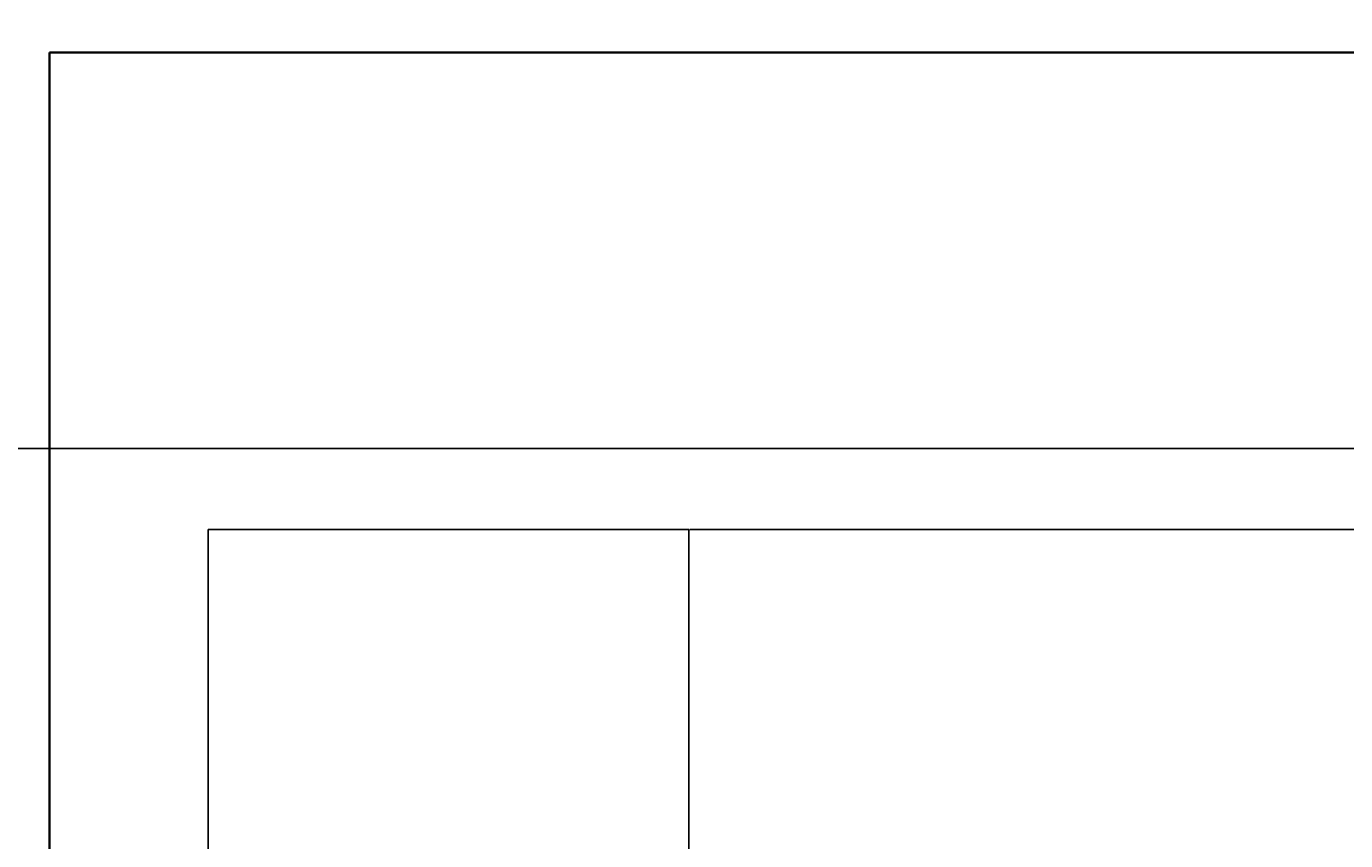
# Model space of a CAD drawing. Units: inches. Extents: x -13 to 809, y 112 to 656.
# Tile 15 of 55: x 111 to 210, y 385 to 446. Entities that reach past the tile are written whole.
import ezdxf

# ---------------------------------------------------------------- set-up
doc = ezdxf.new("R2010")
doc.units = ezdxf.units.IN
doc.header["$MEASUREMENT"] = 0
for name, color, linetype, lineweight in [('A-ANNO-DIMS', 2, 'Continuous', 18), ('A-DOOR', 4, 'Continuous', 25), ('A-ELEV', 7, 'Continuous', 35)]:
    doc.layers.add(name, color=color, linetype=linetype, lineweight=lineweight)
doc.styles.get("Standard").update_dxf_attribs({"font": 'arial.ttf'})
doc.dimstyles.get("Standard").update_dxf_attribs({"dimtxt": 0.625, "dimasz": 0.18, "dimexe": 0.18, "dimexo": 0.0625, "dimgap": 0.09, "dimtad": 0, "dimtih": 1, "dimtoh": 1, "dimdec": 4, "dimzin": 0, "dimdsep": 46, "dimlunit": 4, "dimtxsty": 'Standard', "dimcen": 0.09, "dimadec": 0, "dimazin": 0, "dimtfac": 1, "dimtdec": 4, "dimtofl": 0, "dimtmove": 0, "dimatfit": 3, "dimfxl": 1, "dimtolj": 1, "dimtzin": 0, "dimarcsym": 0})

# ---------------------------------------------------------------- blocks, each defined once
blk = doc.blocks.new('*D39')
at = {"layer": 'A-ANNO-DIMS', "color": 0, "lineweight": -2, "transparency": 16777216}
for p, q in [((341.345, 524.281), (-12.099, 524.281)), ((-11.919, 524.101), (-11.919, 406.775)), ((-11.919, 288.631), (-11.919, 405.957)), ((341.345, 288.451), (-12.099, 288.451))]:
    blk.add_line(p, q, dxfattribs=at)
at = {"layer": 'A-ANNO-DIMS', "color": 0, "transparency": 16777216}
for points in [[(-11.949, 524.101), (-11.889, 524.101), (-11.919, 524.281)], [(-11.949, 288.631), (-11.889, 288.631), (-11.919, 288.451)]]:
    blk.add_solid(points, dxfattribs=at)
at = {"layer": 'Defpoints', "color": 0, "transparency": 16777216}
for p in [(-11.919, 524.281), (341.407, 524.281), (341.407, 288.451)]:
    blk.add_point(p, dxfattribs=at)
at = {"layer": 'A-ANNO-DIMS', "color": 0, "transparency": 16777216, "insert": (-11.919, 406.366), "char_height": 0.625, "attachment_point": 5}
blk.add_mtext('\\A1;235.83', dxfattribs=at)
blk = doc.blocks.new('*D42')
at = {"layer": 'A-ANNO-DIMS', "color": 0, "lineweight": -2, "transparency": 16777216}
for p, q in [((471.037, 414.859), (-12.099, 414.859)), ((-11.919, 414.679), (-11.919, 386.829)), ((-11.919, 358.16), (-11.919, 386.011)), ((471.037, 357.98), (-12.099, 357.98))]:
    blk.add_line(p, q, dxfattribs=at)
at = {"layer": 'A-ANNO-DIMS', "color": 0, "transparency": 16777216}
for points in [[(-11.949, 414.679), (-11.889, 414.679), (-11.919, 414.859)], [(-11.949, 358.16), (-11.889, 358.16), (-11.919, 357.98)]]:
    blk.add_solid(points, dxfattribs=at)
at = {"layer": 'Defpoints', "color": 0, "transparency": 16777216}
for p in [(-11.919, 414.859), (471.1, 414.859), (471.1, 357.98)]:
    blk.add_point(p, dxfattribs=at)
at = {"layer": 'A-ANNO-DIMS', "color": 0, "transparency": 16777216, "insert": (-11.919, 386.42), "char_height": 0.625, "attachment_point": 5}
blk.add_mtext('\\A1;56.88', dxfattribs=at)
blk = doc.blocks.new('*D43')
at = {"layer": 'A-ANNO-DIMS', "color": 0, "lineweight": -2, "transparency": 16777216}
for p, q in [((471.037, 470.877), (-12.099, 470.877)), ((-11.919, 470.697), (-11.919, 443.277)), ((-11.919, 415.039), (-11.919, 442.459)), ((471.037, 414.859), (-12.099, 414.859))]:
    blk.add_line(p, q, dxfattribs=at)
at = {"layer": 'A-ANNO-DIMS', "color": 0, "transparency": 16777216}
for points in [[(-11.949, 470.697), (-11.889, 470.697), (-11.919, 470.877)], [(-11.949, 415.039), (-11.889, 415.039), (-11.919, 414.859)]]:
    blk.add_solid(points, dxfattribs=at)
at = {"layer": 'Defpoints', "color": 0, "transparency": 16777216}
for p in [(-11.919, 470.877), (471.1, 470.877), (471.1, 414.859)]:
    blk.add_point(p, dxfattribs=at)
at = {"layer": 'A-ANNO-DIMS', "color": 0, "transparency": 16777216, "insert": (-11.919, 442.868), "char_height": 0.625, "attachment_point": 5}
blk.add_mtext('\\A1;56.02', dxfattribs=at)
blk = doc.blocks.new('*D46')
at = {"layer": 'A-ANNO-DIMS', "color": 0, "lineweight": -2, "transparency": 16777216}
for p, q in [((160.981, 408.794), (807.769, 408.794)), ((807.589, 408.614), (807.589, 367.066)), ((807.589, 324.7), (807.589, 366.248)), ((160.981, 324.52), (807.769, 324.52))]:
    blk.add_line(p, q, dxfattribs=at)
at = {"layer": 'A-ANNO-DIMS', "color": 0, "transparency": 16777216}
for points in [[(807.559, 408.614), (807.619, 408.614), (807.589, 408.794)], [(807.559, 324.7), (807.619, 324.7), (807.589, 324.52)]]:
    blk.add_solid(points, dxfattribs=at)
at = {"layer": 'Defpoints', "color": 0, "transparency": 16777216}
for p in [(160.918, 408.794), (807.589, 408.794), (160.918, 324.52)]:
    blk.add_point(p, dxfattribs=at)
at = {"layer": 'A-ANNO-DIMS', "color": 0, "transparency": 16777216, "insert": (807.589, 366.657), "char_height": 0.625, "attachment_point": 5}
blk.add_mtext('\\A1;84.27', dxfattribs=at)

msp = doc.modelspace()

# ---------------------------------------------------------------- linework, layer by layer
at = {"layer": 'A-DOOR'}
for p, q in [((124.9184, 348.7114), (124.9184, 408.7939)), ((124.9184, 408.7939), (160.9184, 408.7939)), ((160.9184, 408.7939), (160.9184, 348.7114))]:
    msp.add_line(p, q, dxfattribs=at)
at = {"layer": 'A-ELEV'}
for p, q in [((113.0469, 324.5199), (113.0469, 444.5199)), ((113.0469, 444.5199), (319.5074, 444.5199))]:
    msp.add_line(p, q, dxfattribs=at)

# ---------------------------------------------------------------- dimensions: what is measured, and where the dimension line sits
at = {"layer": 'A-ANNO-DIMS'}
for base, p1, p2, picture, middle in [((-11.9191, 524.281), (341.4072, 288.4508), (341.4072, 524.281), '*D39', (-11.9191, 406.3659)), ((-11.9191, 470.8765), (471.0998, 414.8594), (471.0998, 470.8765), '*D43', (-11.9191, 442.8679)), ((-11.9191, 414.8594), (471.0998, 357.9804), (471.0998, 414.8594), '*D42', (-11.9191, 386.4199)), ((807.5888, 408.7939), (160.9184, 324.5199), (160.9184, 408.7939), '*D46', (807.5888, 366.6569))]:
    dim = msp.add_linear_dim(base=base, p1=p1, p2=p2, angle=90, dimstyle='Standard', override={"dimdec": 2, "dimlfac": 1, "dimrnd": 0, "dimzin": 0, "dimdsep": 46, "dimlunit": 2}, dxfattribs=at)
    dim.commit()
    dim.dimension.update_dxf_attribs({"geometry": picture, "text_midpoint": middle})

doc.saveas('drawing.dxf')
